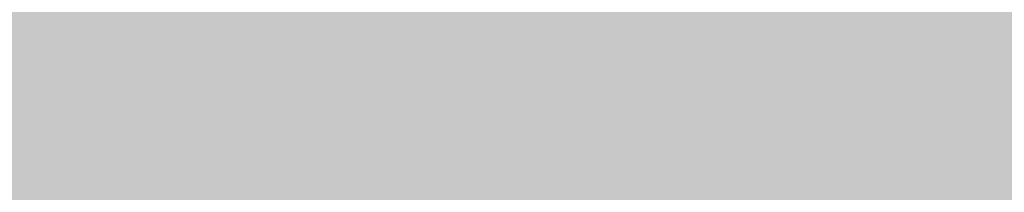
# Model space of a CAD drawing. Units: inches. Extents: x 2091 to 2899, y 967 to 2217.
# Tile 231 of 256: x 2203.4104 to 2203.7172, y 1152.3009 to 1152.3547. Entities that reach past the tile are written whole.
import ezdxf

# ---------------------------------------------------------------- set-up
doc = ezdxf.new("R2010")
doc.units = ezdxf.units.IN
doc.layers.add('A-WALL-PATT', color=141, linetype='Continuous', lineweight=13, true_color=0xadddf7)

msp = doc.modelspace()

# ---------------------------------------------------------------- hatches: boundary and pattern name
at = {"layer": 'A-WALL-PATT'}
h = msp.add_hatch(color=256, dxfattribs=at)
h.dxf.hatch_style = 1
h.paths.add_polyline_path([(2803.1436, 2050.91906), (2203.1436, 2050.91906), (2203.1436, 1090.91906), (2803.1436, 1090.91906)])
h.paths.add_polyline_path([(2635.79885, 1147.54046), (2674.52405, 1147.54046, 0.376086), (2678.52967, 1152.8802), (2678.52967, 1159.55647, 0.333335), (2674.52432, 1163.56185), (2674.52432, 1163.56185), (2674.52432, 1192.93439), (2635.80597, 1192.93439), (2597.08762, 1192.93439), (2597.08762, 1163.56185, 0.333335), (2593.08228, 1159.55647), (2593.08228, 1152.8802, 0.376086), (2597.08789, 1147.54046)], flags=0)
h.paths.add_polyline_path([(2436.01043, 1278.24078, 0.000483), (2435.95264, 1278.21503, -0.001328), (2435.93563, 1278.11169, -0.001711), (2436.11644, 1278.04076, 0.002185)], flags=0)
h.paths.add_polyline_path([(2794.1436, 1143.41906), (2794.1436, 1347.41906), (2543.37017, 1347.41906), (2543.37017, 1351.91906), (2794.1436, 1351.91906), (2794.1436, 1392.71355), (2793.9474, 1392.71355), (2793.9474, 1473.5369), (2794.1436, 1473.5369), (2794.1436, 1531.91906), (2650.1436, 1531.91906), (2650.1436, 1536.41906), (2794.1436, 1536.41906), (2794.1436, 1692.41906), (2609.37561, 1692.41906), (2609.37561, 1644.41906), (2604.87561, 1644.41906), (2604.87561, 1744.91906), (2609.37561, 1744.91906), (2609.37561, 1696.91906), (2794.1436, 1696.91906), (2794.1436, 1780.91906), (2609.6436, 1780.91906), (2493.87561, 1780.91906), (2493.87561, 1785.41906), (2609.6436, 1785.41906), (2794.1436, 1785.41906), (2794.1436, 1847.93882), (2793.95122, 1847.93882), (2793.95122, 1928.76217), (2794.1436, 1928.76217), (2794.1436, 1941.41906), (2614.1436, 1941.41906), (2614.1436, 1821.41906), (2609.6436, 1821.41906), (2609.6436, 1941.41906), (2392.1436, 1941.41906), (2392.1436, 1819.91906), (2387.6436, 1819.91906), (2387.6436, 1941.41906), (2212.1436, 1941.41906), (2212.1436, 1783.91906), (2392.1436, 1783.91906), (2392.1436, 1780.91906), (2212.1436, 1780.91906), (2212.1436, 1629.41906), (2387.6436, 1629.41906), (2387.6436, 1744.91906), (2392.1436, 1744.91906), (2392.1436, 1627.91906), (2317.1436, 1627.91906), (2317.1436, 1551.41906), (2317.1436, 1536.41906), (2459.38359, 1536.41906), (2459.38359, 1602.39648), (2463.88359, 1602.39648), (2463.88359, 1531.91906), (2456.6436, 1531.91906), (2456.6436, 1529.91906), (2452.1436, 1529.91906), (2452.1436, 1531.91906), (2312.6436, 1531.91906), (2312.6436, 1551.41906), (2306.1436, 1551.41906), (2306.1436, 1555.91906), (2308.1436, 1555.91906), (2308.1436, 1551.41906), (2312.6436, 1551.41906), (2312.6436, 1627.91906), (2212.1436, 1627.91906), (2212.1436, 1555.91906), (2270.1436, 1555.91906), (2270.1436, 1551.41906), (2212.1436, 1551.41906), (2212.1436, 1351.91906), (2272.1436, 1351.91906), (2272.1436, 1347.41906), (2212.1436, 1347.41906), (2212.1436, 1275.41906), (2308.1436, 1275.41906), (2308.1436, 1351.91906), (2452.1436, 1351.91906), (2452.1436, 1493.91906), (2456.6436, 1493.91906), (2456.6436, 1347.41906), (2312.6436, 1347.41906), (2312.6436, 1270.91906), (2212.1436, 1270.91906), (2212.1436, 1099.91906), (2281.23752, 1099.91906), (2282.87104, 1110.9138), (2282.00834, 1116.9966), (2278.55774, 1121.4204), (2268.20564, 1128.0562), (2272.08764, 1128.0562), (2273.81294, 1131.927), (2279.42034, 1134.6919), (2285.02784, 1135.2449), (2287.61584, 1137.4568), (2288.04714, 1138.0098), (2289.34114, 1140.7747), (2291.06654, 1139.6687), (2292.36054, 1135.2449), (2295.37984, 1136.9038), (2296.24254, 1135.7979), (2297.10524, 1133.033), (2300.12464, 1138.0098), (2303.14394, 1138.0098), (2304.43794, 1135.7979), (2303.14394, 1133.586), (2306.59464, 1134.6919), (2307.88874, 1133.033), (2310.90804, 1135.2449), (2313.92744, 1134.1389), (2315.62686, 1132.4271), (2308.32004, 1117.5496), (2290.20384, 1109.8079), (2288.90984, 1103.1721), (2289.27231, 1099.91906), (2434.91823, 1099.91906), (2431.59323, 1124.78806), (2429.93023, 1169.55306), (2430.92718, 1240.51969), (2435.65893, 1238.18613), (2437.13523, 1196.55406), (2438.79823, 1143.97306), (2442.67823, 1111.99806), (2446.55823, 1099.91906), (2794.1436, 1099.91906), (2794.1436, 1138.91906), (2548.03245, 1138.91906), (2548.03245, 1143.41906), (2548.03245, 1148.81906), (2546.66846, 1148.03156), (2528.68569, 1179.17862, 0.256256), (2512.03245, 1148.81906), (2512.03245, 1143.41906), (2512.03245, 1138.91906), (2507.53245, 1138.91906), (2507.53245, 1143.41906), (2507.53245, 1148.81906, 0.256256), (2490.8792, 1179.17862), (2472.89644, 1148.03156), (2471.53245, 1148.81906), (2471.53245, 1143.41906), (2467.03245, 1143.41906), (2467.03245, 1269.94579, 0.039061), (2460.90999, 1273.58006), (2467.03245, 1273.58006), (2467.03245, 1286.32536, 0.014511), (2465.21619, 1286.76191), (2467.03245, 1287.05258), (2467.03245, 1323.41906), (2471.53245, 1323.41906), (2471.53245, 1148.81906), (2489.53245, 1179.99597), (2490.89644, 1179.20847), (2490.8792, 1179.17862, -0.256256), (2507.53245, 1148.81906), (2507.53245, 1143.41906), (2512.03245, 1143.41906), (2512.03245, 1148.81906, -0.256256), (2528.68569, 1179.17862), (2528.66846, 1179.20847), (2530.03245, 1179.99597), (2548.03245, 1148.81906), (2548.03245, 1143.41906)], flags=16)
h.paths.add_polyline_path([(2607.76855, 1200.94508), (2607.76855, 1265.03063), (2597.08762, 1281.05201), (2619.78459, 1281.05201), (2627.79528, 1337.12686), (2635.79885, 1337.12686), (2643.81666, 1337.12686), (2651.82736, 1281.05201), (2674.52432, 1281.05201), (2663.8434, 1265.03063), (2663.8434, 1200.94508), (2635.80597, 1200.94508)], flags=0)
edge = h.paths.add_edge_path(flags=0)
edge.add_ellipse((13303.89622, 1272.99872), major_axis=(-10595.31304, 0), ratio=0.84230387009, start_angle=0.628237219, end_angle=0.6465541, ccw=False)
edge.add_ellipse((2711.70045, 1156.85268), major_axis=(2.21977, 0), ratio=0.8423039, start_angle=111.53524, end_angle=180.62824, ccw=False)
edge.add_ellipse((13303.15629, 1272.99872), major_axis=(-10593.02631, 0), ratio=0.84230386954, start_angle=0.528271472, end_angle=0.646554097, ccw=False)
edge.add_line((2710.7646, 1175.3333), (2710.12999, 1175.3333))
edge.add_ellipse((2710.12999, 1176.57978), major_axis=(1.47985, 0), ratio=0.8423039, start_angle=180, end_angle=270, ccw=False)
edge.add_line((2708.65014, 1176.57978), (2708.65014, 1200.78291))
edge.add_ellipse((2710.12999, 1200.78291), major_axis=(1.47985, 0), ratio=0.8423039, start_angle=90, end_angle=180, ccw=False)
edge.add_line((2710.12999, 1202.02939), (2710.46508, 1202.02939))
edge.add_ellipse((13303.15629, 1272.99872), major_axis=(-10593.02631, 0), ratio=0.84230386954, start_angle=-0.090229089, end_angle=0.383866779, ccw=False)
edge.add_ellipse((2710.12999, 1290.92703), major_axis=(-1.47985, 0), ratio=0.8423039, start_angle=0, end_angle=90, ccw=False)
edge.add_line((2708.65014, 1290.92703), (2708.65014, 1315.13017))
edge.add_ellipse((2710.12999, 1315.13017), major_axis=(-1.47985, 0), ratio=0.8423039, start_angle=-90, end_angle=0, ccw=False)
edge.add_line((2710.12999, 1316.37665), (2710.70631, 1316.37665))
edge.add_ellipse((3238.40172, 1296.28957), major_axis=(528.234, 0), ratio=0.84230387, start_angle=176.3495724, end_angle=177.8200497, ccw=False)
edge.add_ellipse((2775.06304, 1071.4507), major_axis=(313.30776, 0), ratio=0.84230387, start_angle=102.1259656, end_angle=103.780529, ccw=False)
edge.add_ellipse((2775.06304, 1078.3057), major_axis=(-305.30289, 0), ratio=0.84230387, start_angle=-79.790461, end_angle=-77.5553727, ccw=False)
edge.add_ellipse((2695.14177, 1541.97538), major_axis=(-250.96022, 0), ratio=0.84230387, start_angle=99.256566, end_angle=102.5549326)
edge.add_line((2741.41033, 1334.21426), (2747.13255, 1337.37848))
edge.add_ellipse((2747.53862, 1336.85748), major_axis=(-0.73992, 0), ratio=0.842304, start_angle=270, end_angle=307.93313, ccw=False)
edge.add_ellipse((2747.53862, 1336.85748), major_axis=(-0.73992, 0), ratio=0.842304, start_angle=232.06687, end_angle=270, ccw=False)
edge.add_line((2747.94469, 1337.37848), (2753.66691, 1334.21426))
edge.add_ellipse((2799.93547, 1541.97538), major_axis=(250.96022, 0), ratio=0.84230387, start_angle=257.4450674, end_angle=260.743434)
edge.add_ellipse((2720.01419, 1078.3057), major_axis=(305.30289, 0), ratio=0.84230387, start_angle=77.5553727, end_angle=79.790461, ccw=False)
edge.add_ellipse((2720.01419, 1071.4507), major_axis=(-313.30776, 0), ratio=0.84230387, start_angle=256.219471, end_angle=257.8740344, ccw=False)
edge.add_ellipse((2256.67551, 1296.28957), major_axis=(-528.234, 0), ratio=0.84230387, start_angle=182.1799503, end_angle=183.6504276, ccw=False)
edge.add_line((2784.37092, 1316.37665), (2784.94725, 1316.37665))
edge.add_ellipse((2784.94725, 1315.13017), major_axis=(1.47985, 0), ratio=0.8423039, start_angle=0, end_angle=90, ccw=False)
edge.add_line((2786.42709, 1315.13017), (2786.42709, 1290.92703))
edge.add_ellipse((2784.94725, 1290.92703), major_axis=(1.47985, 0), ratio=0.8423039, start_angle=270, end_angle=360, ccw=False)
edge.add_ellipse((-7808.07906, 1272.99872), major_axis=(10593.02631, 0), ratio=0.84230386954, start_angle=-0.383866779, end_angle=0.090229089, ccw=False)
edge.add_line((2784.61216, 1202.02939), (2784.94725, 1202.02939))
edge.add_ellipse((2784.94725, 1200.78291), major_axis=(1.47985, 0), ratio=0.8423039, start_angle=0, end_angle=90, ccw=False)
edge.add_line((2786.42709, 1200.78291), (2786.42709, 1176.57978))
edge.add_ellipse((2784.94725, 1176.57978), major_axis=(-1.47985, 0), ratio=0.8423039, start_angle=90, end_angle=180, ccw=False)
edge.add_line((2784.94725, 1175.3333), (2784.31264, 1175.3333))
edge.add_ellipse((-7808.07906, 1272.99872), major_axis=(10593.02631, 0), ratio=0.84230386954, start_angle=-0.618643196, end_angle=-0.528271472, ccw=False)
edge.add_ellipse((2783.37678, 1156.85268), major_axis=(-2.21977, 0), ratio=0.8423039, start_angle=179.37176, end_angle=248.46476, ccw=False)
edge.add_ellipse((-7808.81898, 1272.99872), major_axis=(-10595.31304, 0), ratio=0.84230386576, start_angle=179.353445923, end_angle=179.371762803, ccw=False)
edge.add_ellipse((2780.2973, 1153.50079), major_axis=(-5.24643, 0), ratio=0.8423039, start_angle=90, end_angle=179.35345, ccw=False)
edge.add_line((2780.2973, 1149.08171), (2714.77993, 1149.08171))
edge.add_ellipse((2714.77993, 1153.50079), major_axis=(5.24643, 0), ratio=0.8423039, start_angle=180.64655, end_angle=270, ccw=False)
edge = h.paths.add_edge_path(flags=0)
edge.add_line((2718.18737, 1151.00783), (2718.18737, 1170.47236))
edge.add_ellipse((2721.14706, 1170.47236), major_axis=(-2.95969, 0), ratio=0.8423039, start_angle=-90, end_angle=0, ccw=False)
edge.add_line((2721.14706, 1172.96532), (2773.93017, 1172.96532))
edge.add_ellipse((2773.93017, 1170.47236), major_axis=(-2.95969, 0), ratio=0.8423039, start_angle=180, end_angle=270, ccw=False)
edge.add_line((2776.88987, 1170.47236), (2776.88987, 1151.00783))
edge.add_line((2776.88987, 1151.00783), (2718.18737, 1151.00783))
edge = h.paths.add_edge_path(flags=0)
edge.add_line((2718.18737, 1180.23415), (2718.18737, 1199.05783))
edge.add_ellipse((2747.53862, 1320.39864), major_axis=(147.01792, 0), ratio=0.84230387, start_angle=256.4018653, end_angle=283.5981347)
edge.add_line((2776.88987, 1199.05783), (2776.88987, 1180.23415))
edge.add_ellipse((2747.53862, 1301.57496), major_axis=(147.01792, 0), ratio=0.84230387, start_angle=256.4018653, end_angle=283.5981347, ccw=False)
edge = h.paths.add_edge_path(flags=0)
edge.add_ellipse((13303.15629, 1272.99872), major_axis=(-10591.54646, 0), ratio=0.84230386955, start_angle=0.055594314, end_angle=0.377764194, ccw=False)
edge.add_line((2711.61686, 1262.72171), (2715.66741, 1249.4954))
edge.add_ellipse((6413.89196, 1241.69192), major_axis=(-3698.23616, 0), ratio=0.8423038695, start_angle=-0.12089737, end_angle=0.36407635)
edge.add_line((2715.76104, 1218.19245), (2711.93431, 1203.16736))
edge = h.paths.add_edge_path(flags=0)
edge.add_line((2718.18737, 1251.07457), (2716.00249, 1267.45044))
edge.add_ellipse((2742.15117, 1202.18954), major_axis=(81.77258, 0), ratio=0.84230387, start_angle=94.277421, end_angle=111.8349538, ccw=False)
edge.add_line((2737.00975, 1270.93063), (2758.06748, 1270.93063))
edge.add_ellipse((2752.92606, 1202.18954), major_axis=(81.77258, 0), ratio=0.84230387, start_angle=68.1650462, end_angle=85.722579, ccw=False)
edge.add_line((2779.07475, 1267.45044), (2776.88987, 1251.07457))
edge.add_ellipse((2750.33806, 1187.88536), major_axis=(79.57966, 0), ratio=0.84230387, start_angle=67.2080851, end_angle=85.1299304)
edge.add_line((2756.03466, 1254.74366), (2739.04258, 1254.74366))
edge.add_ellipse((2744.73917, 1187.88536), major_axis=(79.57966, 0), ratio=0.84230387, start_angle=94.8700696, end_angle=112.7919149)
edge = h.paths.add_edge_path(flags=0)
edge.add_line((2783.14293, 1203.16736), (2779.31619, 1218.19245))
edge.add_ellipse((-918.81473, 1241.69192), major_axis=(3698.23616, 0), ratio=0.8423038695, start_angle=-0.36407635, end_angle=0.12089737)
edge.add_line((2779.40983, 1249.4954), (2783.46037, 1262.72171))
edge.add_ellipse((-7808.07906, 1272.99872), major_axis=(-10591.54646, 0), ratio=0.84230386954, start_angle=179.622235806, end_angle=179.944405687, ccw=False)
edge = h.paths.add_edge_path(flags=0)
edge.add_ellipse((2734.20089, 1286.69044), major_axis=(-0.35661, 6.34008), ratio=0.6038336, start_angle=89.002014, end_angle=253.657408, ccw=False)
edge.add_line((2730.369, 1286.54181), (2730.369, 1301.35198))
edge.add_line((2730.369, 1301.35198), (2735.91331, 1305.2148))
edge.add_ellipse((2736.38492, 1304.73456), major_axis=(0.73992, 0), ratio=0.842304, start_angle=90, end_angle=134.48021, ccw=False)
edge.add_line((2736.38492, 1305.3578), (2738.03278, 1305.3578))
edge.add_line((2738.03278, 1305.3578), (2738.03278, 1307.70793))
edge.add_ellipse((2794.20164, 1307.70793), major_axis=(56.16886, 0), ratio=0.84230387, start_angle=150.56143, end_angle=180, ccw=False)
edge.add_ellipse((2700.87559, 1307.70793), major_axis=(-56.16886, 0), ratio=0.84230387, start_angle=180, end_angle=209.43857, ccw=False)
edge.add_line((2757.04445, 1307.70793), (2757.04445, 1305.3578))
edge.add_line((2757.04445, 1305.3578), (2758.69232, 1305.3578))
edge.add_ellipse((2758.69232, 1304.73456), major_axis=(-0.73992, 0), ratio=0.842304, start_angle=225.51979, end_angle=270, ccw=False)
edge.add_line((2759.16392, 1305.2148), (2764.70823, 1301.35198))
edge.add_line((2764.70823, 1301.35198), (2764.70823, 1286.54181))
edge.add_ellipse((2760.87634, 1286.69044), major_axis=(0.35661, 6.34008), ratio=0.6038336, start_angle=106.342592, end_angle=270.997986, ccw=False)
edge.add_line((2757.04445, 1285.79709), (2757.04445, 1307.70793))
edge.add_ellipse((2700.87559, 1307.70793), major_axis=(-56.16886, 0), ratio=0.84230387, start_angle=180, end_angle=209.43857)
edge.add_ellipse((2794.20164, 1307.70793), major_axis=(56.16886, 0), ratio=0.84230387, start_angle=150.56143, end_angle=180)
edge.add_line((2738.03278, 1307.70793), (2738.03278, 1285.79709))
h.paths.add_polyline_path([(2417.81227, 1104.4497), (2413.49227, 1102.5297), (2410.61227, 1103.9697), (2409.17227, 1106.3697), (2407.25227, 1107.3297), (2406.29227, 1109.7297), (2405.33227, 1114.0497), (2405.33227, 1117.8897), (2406.29227, 1120.1297), (2407.25227, 1119.8097), (2408.84832, 1118.32766), (2410.17395, 1119.42417), (2410.21127, 1120.4057), (2411.04073, 1121.41905), (2410.69927, 1119.8587), (2410.17395, 1119.42417), (2410.08845, 1117.17611), (2411.13284, 1116.20632), (2413.97227, 1119.3297), (2416.85227, 1120.7697), (2416.86972, 1120.79878), (2417.03507, 1119.40512), (2417.89621, 1118.14338), (2418.29227, 1118.3697), (2419.54445, 1120.03927), (2419.36092, 1118.38749), (2419.03211, 1119.35615), (2418.39894, 1118.51193), (2419.25227, 1114.5297), (2418.79409, 1107.19879)], flags=0)
h.paths.add_polyline_path([(2508.87017, 1347.41906), (2508.37017, 1347.41906), (2508.37017, 1351.91906), (2508.87017, 1351.91906)], flags=0)
h.paths.add_polyline_path([(2473.37017, 1347.41906), (2472.37017, 1347.41906), (2467.87017, 1347.41906), (2467.87017, 1455.41906), (2472.37017, 1455.41906), (2472.37017, 1352.41906), (2473.37017, 1352.41906)], flags=0)
h.paths.add_polyline_path([(2352.10624, 1217.4462), (2349.22624, 1218.8862), (2347.78624, 1221.2862), (2345.86624, 1222.2462), (2344.90624, 1224.6462), (2343.94624, 1228.9662), (2343.94624, 1232.8062), (2344.90624, 1235.0462), (2345.86624, 1234.7262), (2347.46229, 1233.24415), (2348.78792, 1234.34066), (2348.82524, 1235.3222), (2349.6547, 1236.33555), (2349.31324, 1234.7752), (2348.78792, 1234.34066), (2348.70242, 1232.0926), (2349.74681, 1231.12282), (2352.58624, 1234.2462), (2355.46624, 1235.6862), (2355.48369, 1235.71528), (2355.64904, 1234.32161), (2356.51018, 1233.05988), (2356.90624, 1233.2862), (2358.15842, 1234.95576), (2357.97489, 1233.30398), (2357.64608, 1234.27264), (2357.01291, 1233.42842), (2357.86624, 1229.4462), (2357.40806, 1222.11529), (2356.42624, 1219.3662)], flags=0)
h.paths.add_polyline_path([(2348.2968, 1112.22442), (2347.0138, 1112.31042), (2345.5298, 1114.12742), (2345.7318, 1115.85842), (2346.8118, 1116.98242), (2346.8118, 1114.64642), (2345.8668, 1114.21442), (2346.8798, 1114.30042)], flags=0)
h.paths.add_polyline_path([(2347.0138, 1110.92642), (2346.2718, 1110.49342), (2346.6098, 1111.18642)], flags=0)
h.paths.add_polyline_path([(2345.8668, 1118.19442), (2345.5298, 1117.32942), (2343.7078, 1118.02142), (2344.3828, 1118.62642)], flags=0)
h.paths.add_polyline_path([(2346.6768, 1109.28242), (2346.0698, 1108.07142), (2345.8668, 1110.06142)], flags=0)
h.paths.add_polyline_path([(2345.0568, 1119.75142), (2343.6398, 1119.75142), (2343.9778, 1121.13542)], flags=0)
h.paths.add_polyline_path([(2345.2598, 1116.55042), (2345.1248, 1115.85842), (2344.9218, 1115.68542), (2344.7198, 1116.37742)], flags=0)
h.paths.add_polyline_path([(2345.6648, 1112.31042), (2345.4618, 1111.53242), (2344.0448, 1111.96442), (2344.6518, 1112.57042)], flags=0)
h.paths.add_polyline_path([(2345.1918, 1113.34942), (2344.4498, 1113.86842), (2344.7198, 1114.38742)], flags=0)
h.paths.add_polyline_path([(2344.6518, 1116.80942), (2344.1798, 1115.68542), (2344.6518, 1115.33942), (2343.9098, 1114.90642), (2343.0328, 1115.94442), (2343.6398, 1116.46342)], flags=0)
h.paths.add_polyline_path([(2345.8668, 1106.68642), (2344.9898, 1105.56242), (2344.5168, 1106.60042)], flags=0)
h.paths.add_polyline_path([(2344.8548, 1110.06142), (2344.5168, 1109.28242), (2344.1128, 1109.71542)], flags=0)
h.paths.add_polyline_path([(2344.0448, 1113.52242), (2343.4378, 1113.08942), (2342.7628, 1113.95442)], flags=0)
h.paths.add_polyline_path([(2344.3148, 1111.01242), (2342.9648, 1110.32042), (2342.9648, 1111.09942)], flags=0)
h.paths.add_polyline_path([(2345.1248, 1104.69742), (2344.5848, 1103.74542), (2344.4498, 1104.26442)], flags=0)
h.paths.add_polyline_path([(2342.8298, 1121.22242), (2341.7498, 1120.53042), (2340.5358, 1121.04942), (2340.1308, 1121.82842), (2340.6708, 1122.95242), (2341.1428, 1121.82842), (2341.6148, 1122.00142)], flags=0)
h.paths.add_polyline_path([(2342.9648, 1119.75142), (2343.0328, 1118.45342), (2342.0878, 1118.02142), (2342.0198, 1119.49142)], flags=0)
h.paths.add_polyline_path([(2342.6948, 1116.89642), (2341.9528, 1116.63642), (2342.0198, 1117.32942)], flags=0)
h.paths.add_polyline_path([(2343.0328, 1112.22442), (2342.0198, 1111.79142), (2341.5478, 1112.22442), (2342.3578, 1113.34942)], flags=0)
h.paths.add_polyline_path([(2343.7748, 1104.43742), (2342.6278, 1102.88042), (2342.6948, 1104.61042), (2343.4378, 1105.12942)], flags=0)
h.paths.add_polyline_path([(2342.0198, 1115.07942), (2340.8058, 1115.51242), (2340.9408, 1116.37742)], flags=0)
h.paths.add_polyline_path([(2341.4808, 1120.09742), (2341.4808, 1119.40542), (2341.0758, 1119.57842), (2341.1428, 1120.09742)], flags=0)
h.paths.add_polyline_path([(2341.8178, 1114.47342), (2340.9408, 1113.08942), (2340.8058, 1114.56042)], flags=0)
h.paths.add_polyline_path([(2341.1428, 1118.54042), (2340.9408, 1116.98242), (2339.0508, 1117.67542), (2339.0508, 1118.62642)], flags=0)
h.paths.add_polyline_path([(2342.6948, 1101.66842), (2341.9528, 1101.84142), (2342.5598, 1102.36142)], flags=0)
h.paths.add_polyline_path([(2340.3328, 1119.66542), (2338.4438, 1119.57842), (2337.9038, 1120.35742), (2339.6578, 1120.61642)], flags=0)
h.paths.add_polyline_path([(2340.3328, 1115.33942), (2340.0628, 1113.69542), (2339.3878, 1115.33942)], flags=0)
h.paths.add_polyline_path([(2341.8178, 1103.83142), (2341.5478, 1102.88042), (2341.1428, 1103.65842)], flags=0)
h.paths.add_polyline_path([(2339.0508, 1122.86642), (2337.2958, 1121.82842), (2337.0938, 1123.12542), (2337.7688, 1123.81842)], flags=0)
h.paths.add_polyline_path([(2339.1178, 1121.74142), (2338.8478, 1121.22242), (2338.1738, 1121.04942), (2338.3758, 1121.56842)], flags=0)
h.paths.add_polyline_path([(2339.1858, 1119.31942), (2338.6458, 1118.71342), (2338.2408, 1118.10742), (2338.2408, 1118.88642)], flags=0)
h.paths.add_polyline_path([(2341.1428, 1101.92842), (2340.6028, 1101.23642), (2340.0628, 1101.84142), (2340.6028, 1102.36142)], flags=0)
h.paths.add_polyline_path([(2337.6338, 1117.76142), (2336.6208, 1118.28042), (2337.2958, 1118.97242)], flags=0)
h.paths.add_polyline_path([(2336.8238, 1119.57842), (2334.7988, 1118.97242), (2335.2038, 1120.35742), (2336.5538, 1120.87642)], flags=0)
h.paths.add_polyline_path([(2339.1178, 1100.45742), (2337.3638, 1100.54342), (2336.7558, 1101.23642)], flags=0)
h.paths.add_polyline_path([(2336.3508, 1122.43342), (2336.0138, 1121.91442), (2334.9338, 1122.43342), (2334.5288, 1123.47142), (2335.7438, 1122.77942)], flags=0)
h.paths.add_polyline_path([(2334.7318, 1120.87642), (2334.2588, 1120.35742), (2334.0568, 1120.78942), (2334.5968, 1121.30842)], flags=0)
h.paths.add_polyline_path([(2334.4618, 1122.17442), (2332.5718, 1121.30842), (2331.3568, 1122.17442), (2332.0998, 1122.86642)], flags=0)
h.paths.add_polyline_path([(2334.2588, 1118.54042), (2333.3818, 1118.45342), (2333.6518, 1119.31942)], flags=0)
h.paths.add_polyline_path([(2335.5418, 1102.27442), (2334.1918, 1102.62042), (2335.2718, 1103.31242)], flags=0)
h.paths.add_polyline_path([(2332.7068, 1119.66542), (2331.6948, 1120.44342), (2332.5048, 1120.78942)], flags=0)
h.paths.add_polyline_path([(2334.7318, 1101.14942), (2333.5168, 1101.58242), (2333.9888, 1101.75542)], flags=0)
h.paths.add_polyline_path([(2332.6398, 1116.63642), (2331.0868, 1116.29042), (2331.9648, 1118.19442)], flags=0)
h.paths.add_polyline_path([(2330.7498, 1121.56842), (2330.2768, 1120.27042), (2328.5228, 1119.31942), (2328.9948, 1121.04942)], flags=0)
h.paths.add_polyline_path([(2330.7498, 1118.62642), (2330.0078, 1117.50242), (2329.8728, 1118.02142)], flags=0)
h.paths.add_polyline_path([(2332.0998, 1102.36142), (2330.5468, 1102.01442), (2331.6948, 1102.96642)], flags=0)
h.paths.add_polyline_path([(2329.5348, 1113.60842), (2329.0628, 1112.31042), (2328.5898, 1113.34942)], flags=0)
h.paths.add_polyline_path([(2328.3878, 1117.84842), (2327.5098, 1116.55042), (2327.1728, 1117.76142)], flags=0)
h.paths.add_polyline_path([(2329.7378, 1106.51342), (2329.5348, 1105.30242), (2328.2528, 1106.08142)], flags=0)
h.paths.add_polyline_path([(2328.6578, 1114.38742), (2328.0498, 1114.12742), (2328.3198, 1114.90642)], flags=0)
h.paths.add_polyline_path([(2328.3198, 1112.22442), (2327.1058, 1112.13742), (2326.7008, 1112.65642)], flags=0)
h.paths.add_polyline_path([(2326.9028, 1115.25242), (2326.7008, 1114.12742), (2325.2158, 1113.60842), (2326.0928, 1115.33942)], flags=0)
h.paths.add_polyline_path([(2326.6328, 1108.33042), (2326.0928, 1107.37942), (2325.8908, 1108.50342), (2326.4978, 1109.10942)], flags=0)
h.paths.add_polyline_path([(2615.1436, 1531.91906), (2609.6436, 1531.91906), (2609.6436, 1620.41906), (2614.1436, 1620.41906), (2614.1436, 1536.41906), (2615.1436, 1536.41906)], flags=0)
h.paths.add_polyline_path([(2545.1436, 1563.41906), (2464.1436, 1563.41906), (2464.1436, 1632.41906), (2509.1436, 1632.41906), (2509.1436, 1627.91906), (2509.1436, 1603.91906), (2468.6436, 1603.91906), (2468.6436, 1567.91906), (2540.6436, 1567.91906), (2540.6436, 1591.91906), (2545.1436, 1591.91906)], flags=0)
h.paths.add_polyline_path([(2388.96905, 1549.98573), (2357.43418, 1549.98573), (2357.43418, 1623.36078), (2399.36278, 1623.36078), (2435.68947, 1623.36078), (2435.59255, 1602.55927), (2435.59255, 1602.39648), (2388.96905, 1602.39648)], flags=0)
h.paths.add_polyline_path([(2388.88063, 1555.80915), (2374.90443, 1555.80915), (2374.90443, 1600.57156), (2374.90443, 1615.45765), (2406.35088, 1615.45765), (2406.35088, 1618.93943), (2412.17429, 1615.45765), (2406.35088, 1611.97586), (2406.35088, 1615.45765), (2388.88063, 1615.45765)], flags=0)
h.paths.add_polyline_path([(2568.87561, 1644.41906), (2453.37561, 1644.41906), (2453.37561, 1785.41906), (2457.87561, 1785.41906), (2457.87561, 1648.91906), (2568.87561, 1648.91906)], flags=0)
h.paths.add_polyline_path([(2212.1436, 1945.91906), (2212.1436, 2041.91906), (2794.1436, 2041.91906), (2794.1436, 1945.91906)], flags=16)
h.paths.add_polyline_path([(2271.08273, 1964.31724), (2776.85297, 1964.31724), (2776.85297, 2037.16962), (2271.08273, 2037.16962)], flags=8)
h.paths.add_polyline_path([(2380.64929, 1536.82414), (2461.04081, 1536.82414), (2461.04081, 1554.65259), (2380.64929, 1554.65259)], flags=8)
h.paths.add_polyline_path([(2240.75571, 1609.72545), (2309.18583, 1609.72545), (2309.18583, 1617.6982), (2240.75571, 1617.6982)], flags=8)
h.paths.add_polyline_path([(2212.67726, 1313.5041), (2282.59152, 1313.5041), (2282.59152, 1322.74524), (2212.67726, 1322.74524)], flags=8)
h.paths.add_polyline_path([(2457.11198, 1114.77857), (2558.48158, 1114.77857), (2558.48158, 1142.21968), (2457.11198, 1142.21968)], flags=8)
h.paths.add_polyline_path([(2473.44234, 1273.01007), (2604.64123, 1273.01007), (2604.64123, 1318.34693), (2473.44234, 1318.34693)], flags=8)
h.paths.add_polyline_path([(2638.8763, 1626.97743), (2684.25037, 1627.97674), (2684.03848, 1637.59749), (2638.66442, 1636.59819)], flags=8)
h.paths.add_polyline_path([(2537.59055, 1453.79345), (2628.38955, 1453.79345), (2628.38955, 1475.34481), (2537.59055, 1475.34481)], flags=8)
h.paths.add_polyline_path([(2504.13764, 1714.6324), (2554.64719, 1714.6324), (2554.64719, 1730.23771), (2504.13764, 1730.23771)], flags=8)
h.paths.add_polyline_path([(2487.50118, 1575.65187), (2535.09712, 1575.65187), (2535.09712, 1598.37765), (2487.50118, 1598.37765)], flags=8)
h.paths.add_polyline_path([(2709.0994, 1735.71028), (2740.0166, 1735.71028), (2740.0166, 1749.93764), (2709.0994, 1749.93764)], flags=8)
h.paths.add_polyline_path([(2442.43842, 1792.17166), (2564.72884, 1792.17166), (2564.72884, 1842.00016), (2442.43842, 1842.00016)], flags=8)
h.paths.add_polyline_path([(2655.8158, 1809.64408), (2789.52014, 1806.6938), (2790.08498, 1832.29164), (2656.38064, 1835.24192)], flags=8)
h.paths.add_polyline_path([(2234.8427, 1797.72014), (2368.59285, 1794.76885), (2369.16072, 1820.50413), (2235.41056, 1823.45542)], flags=8)
h.paths.add_polyline_path([(2245.13847, 1644.00633), (2398.42773, 1640.6239), (2398.99484, 1666.32482), (2245.70557, 1669.70725)], flags=8)
h.paths.add_polyline_path([(2306.14285, 1431.16852), (2413.76831, 1428.79369), (2414.33315, 1454.39153), (2306.70768, 1456.76636)], flags=8)
h.paths.add_polyline_path([(2306.83458, 1458.23314), (2393.38048, 1456.32345), (2393.93281, 1481.35436), (2307.38691, 1483.26405)], flags=8)

doc.saveas('drawing.dxf')
